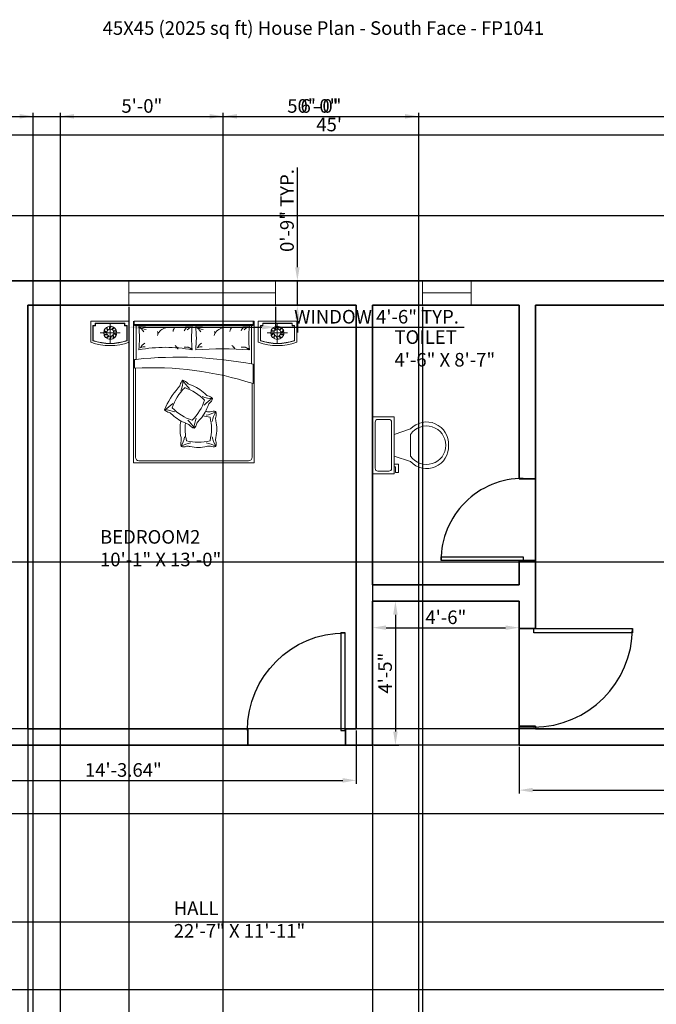
# Model space of a CAD drawing. Units: inches. Extents: x -938 to -211, y -366 to 366.
# Tile 3 of 4: x -684 to -450, y 4 to 366. Entities that reach past the tile are written whole.
import ezdxf

# ---------------------------------------------------------------- set-up
doc = ezdxf.new("R2010")
doc.units = ezdxf.units.IN
doc.header["$PDMODE"] = 35
doc.header["$PDSIZE"] = 5
for name, color, linetype, lineweight in [('A-ANNO-DIMS', 2, 'Continuous', 18), ('A-AREA-IDEN', 7, 'Continuous', 18), ('A-DOOR', 3, 'Continuous', 25), ('A-FLOR-FIXT', 9, 'Continuous', 18), ('A-GLAZ', 4, 'Continuous', 18), ('A-WALL', 7, 'Continuous', 35), ('C-PROP', 8, 'Continuous', 25), ('furn', 28, 'Continuous', 13), ('txt', 7, 'Continuous', 18)]:
    doc.layers.add(name, color=color, linetype=linetype, lineweight=lineweight)
doc.styles.get("Standard").update_dxf_attribs({"font": 'arial.ttf'})
doc.dimstyles.new('ISO-25', dxfattribs={"dimtxt": 5, "dimasz": 5, "dimexe": 1.25, "dimexo": 0.625, "dimtad": 1, "dimlunit": 3, "dimtxsty": 'Standard', "dimcen": 2.5, "dimadec": 0, "dimazin": 0, "dimtfac": 1, "dimtmove": 0, "dimatfit": 3, "dimfxl": 1, "dimarcsym": 0})

# ---------------------------------------------------------------- blocks, each defined once
blk = doc.blocks.new('*U2')
for p, q in [((0, 0), (0, -6)), ((40, 0), (40, -6))]:
    blk.add_line(p, q)
blk.add_lwpolyline([(0, 0), (0, 40), (1.75, 40), (1.75, 0)], close=True)
blk.add_arc((0, 0), 40, 0, 90)
blk = doc.blocks.new('*U4')
for p, q in [((9.5, -6), (9.5, -2)), ((-10, -8.5), (-8, -8.5)), ((-10, -9.5), (-10, -8.5)), ((-7, -9.5), (-10, -9.5)), ((-8, -8.5), (-8, -8)), ((-7, -8), (-7, -9.5)), ((-4, -8), (-6, -14)), ((4, -8), (6, -14)), ((4, -14), (-4, -14))]:
    blk.add_line(p, q)
blk.add_lwpolyline([(10.5, -8), (10.5, 0), (-10.5, 0), (-10.5, -8)], close=True)
for points in [[(-9.5, -2), (-9.5, -6)], [(8.5, -1), (-8.5, -1)], [(-8.5, -7), (8.5, -7)]]:
    blk.add_lwpolyline(points)
for centre, radius, start, end in [((-8.625, -1.875), 0.8839, 81.8699, 188.1301), ((8.625, -1.875), 0.8839, 351.8699, 98.1301), ((-8.625, -6.125), 0.8839, 171.869898, 278.1301), ((8.625, -6.125), 0.8839, 261.8699, 8.1301), ((-0.4772, -19.9188), 8.0953, 133.01722, 273.38), ((0.0374, -19.8731), 7.127, 124.50543, 269.7), ((-0.0373, -19.8731), 7.127, 270.3, 55.4946), ((0.4773, -19.9188), 8.0953, 266.62, 46.9828)]:
    blk.add_arc(centre, radius, start, end)
blk = doc.blocks.new('*D7')
at = {"layer": 'A-ANNO-DIMS', "color": 0, "lineweight": -2, "transparency": 16777216}
for p, q in [((-554.06, 151.36), (-554.06, 140.97)), ((-500.06, 151.36), (-500.06, 140.97)), ((-549.06, 142.22), (-505.06, 142.22))]:
    blk.add_line(p, q, dxfattribs=at)
at = {"layer": 'A-ANNO-DIMS', "color": 0, "transparency": 16777216}
for points in [[(-549.06, 143.05), (-549.06, 141.39), (-554.06, 142.22)], [(-505.06, 143.05), (-505.06, 141.39), (-500.06, 142.22)]]:
    blk.add_solid(points, dxfattribs=at)
at = {"layer": 'Defpoints', "color": 0, "transparency": 16777216}
for p in [(-554.06, 151.98), (-500.06, 151.98), (-500.06, 142.22)]:
    blk.add_point(p, dxfattribs=at)
at = {"layer": 'A-ANNO-DIMS', "color": 0, "transparency": 16777216, "insert": (-527.06, 145.4), "char_height": 5, "attachment_point": 5}
blk.add_mtext('4\'-6"', dxfattribs=at)
blk = doc.blocks.new('*D8')
at = {"layer": 'A-ANNO-DIMS', "color": 0, "lineweight": -2, "transparency": 16777216}
for p, q in [((-553.44, 151.98), (-544.39, 151.98)), ((-545.64, 146.98), (-545.64, 103.98)), ((-553.44, 98.98), (-544.39, 98.98))]:
    blk.add_line(p, q, dxfattribs=at)
at = {"layer": 'A-ANNO-DIMS', "color": 0, "transparency": 16777216}
for points in [[(-546.47, 146.98), (-544.8, 146.98), (-545.64, 151.98)], [(-546.47, 103.98), (-544.8, 103.98), (-545.64, 98.98)]]:
    blk.add_solid(points, dxfattribs=at)
at = {"layer": 'Defpoints', "color": 0, "transparency": 16777216}
for p in [(-554.06, 151.98), (-554.06, 98.98), (-545.64, 98.98)]:
    blk.add_point(p, dxfattribs=at)
at = {"layer": 'A-ANNO-DIMS', "color": 0, "transparency": 16777216, "insert": (-548.8, 125.48), "char_height": 5, "attachment_point": 5, "rotation": 90}
blk.add_mtext('4\'-5"', dxfattribs=at)
blk = doc.blocks.new('*D9')
at = {"layer": 'A-ANNO-DIMS', "color": 0, "lineweight": -2, "transparency": 16777216}
for p, q in [((-500.06, 98.36), (-500.06, 81.14)), ((-309.06, 98.36), (-309.06, 81.14)), ((-495.06, 82.39), (-314.06, 82.39))]:
    blk.add_line(p, q, dxfattribs=at)
at = {"layer": 'A-ANNO-DIMS', "color": 0, "transparency": 16777216}
for points in [[(-495.06, 83.22), (-495.06, 81.55), (-500.06, 82.39)], [(-314.06, 83.22), (-314.06, 81.55), (-309.06, 82.39)]]:
    blk.add_solid(points, dxfattribs=at)
at = {"layer": 'Defpoints', "color": 0, "transparency": 16777216}
for p in [(-500.06, 98.98), (-309.06, 98.98), (-309.06, 82.39)]:
    blk.add_point(p, dxfattribs=at)
at = {"layer": 'A-ANNO-DIMS', "color": 0, "transparency": 16777216, "insert": (-404.56, 85.56), "char_height": 5, "attachment_point": 5}
blk.add_mtext('15\'-11"', dxfattribs=at)
blk = doc.blocks.new('*D14')
at = {"layer": 'A-ANNO-DIMS', "color": 0, "lineweight": -2, "transparency": 16777216}
for p, q in [((-560.06, 104.36), (-560.06, 84.74)), ((-731.7, 98.36), (-731.7, 84.74)), ((-726.7, 85.99), (-565.06, 85.99))]:
    blk.add_line(p, q, dxfattribs=at)
at = {"layer": 'A-ANNO-DIMS', "color": 0, "transparency": 16777216}
for points in [[(-726.7, 86.82), (-726.7, 85.15), (-731.7, 85.99)], [(-565.06, 86.82), (-565.06, 85.15), (-560.06, 85.99)]]:
    blk.add_solid(points, dxfattribs=at)
at = {"layer": 'Defpoints', "color": 0, "transparency": 16777216}
for p in [(-560.06, 104.98), (-731.7, 98.98), (-560.06, 85.99)]:
    blk.add_point(p, dxfattribs=at)
at = {"layer": 'A-ANNO-DIMS', "color": 0, "transparency": 16777216, "insert": (-645.88, 89.17), "char_height": 5, "attachment_point": 5}
blk.add_mtext('14\'-3.64"', dxfattribs=at)
blk = doc.blocks.new('*D22')
at = {"layer": 'A-ANNO-DIMS', "color": 0, "lineweight": -2, "transparency": 16777216}
for p, q in [((-840.06, 270.61), (-840.06, 324.96)), ((-835.06, 323.71), (-305.06, 323.71)), ((-300.06, 270.61), (-300.06, 324.96))]:
    blk.add_line(p, q, dxfattribs=at)
at = {"layer": 'A-ANNO-DIMS', "color": 0, "transparency": 16777216}
for points in [[(-835.06, 324.54), (-835.06, 322.87), (-840.06, 323.71)], [(-305.06, 324.54), (-305.06, 322.87), (-300.06, 323.71)]]:
    blk.add_solid(points, dxfattribs=at)
at = {"layer": 'Defpoints', "color": 0, "transparency": 16777216}
for p in [(-300.06, 323.71), (-840.06, 269.98), (-300.06, 269.98)]:
    blk.add_point(p, dxfattribs=at)
at = {"layer": 'A-ANNO-DIMS', "color": 0, "transparency": 16777216, "insert": (-570.06, 326.87), "char_height": 5, "attachment_point": 5}
blk.add_mtext("45'", dxfattribs=at)
blk = doc.blocks.new('BED-DOUBLE-WITH-NIGHTSTANDS')
for p, q in [((-30.77, -7.97), (-30.77, -0.55)), ((-21.46, -1.59), (21.46, -1.59)), ((-21.24, -1.21), (-21.24, -14.04)), ((21.22, -1.21), (21.22, -15.71)), ((30.77, -7.97), (30.77, -0.55)), ((-34.48, -4.26), (-27.06, -4.26)), ((34.48, -4.26), (27.06, -4.26))]:
    blk.add_line(p, q)
for points in [[(-37.91, -7.71), (-37.91, 0), (-23.78, 0), (-23.78, -7.71, -0.181818)], [(-20.26, -10.53, 0.058596), (-20.26, -1.94, 0.036889), (-0.58, -1.94, 0.052163), (-0.58, -10.53, 0.093111)], [(0.7, -10.53, 0.058596), (0.7, -1.94, 0.036648), (20.51, -1.94, 0.052163), (20.51, -10.53, 0.036967)], [(37.91, -7.71), (37.91, 0), (23.78, 0), (23.78, -7.71, 0.181818)], [(-21.84, -14.04), (-21.24, -14.04, -0.072944), (21.82, -15.84), (21.82, -22.97, 0.092568), (-21.84, -17.31)]]:
    blk.add_lwpolyline(points, format="xyb", close=True)
for points in [[(-36.29, -0.77), (-36.29, -1.62), (-37.14, -1.62)], [(-36.22, -0.77), (-36.22, -1.7), (-37.14, -1.7)], [(-36.29, -0.77), (-25.39, -0.77)], [(-36.29, -0.85), (-25.39, -0.85)], [(-25.47, -0.77), (-25.47, -1.7), (-24.55, -1.7)], [(-25.39, -0.77), (-25.39, -1.62), (-24.55, -1.62)], [(-22.23, 0), (-22.23, -52.18), (22.23, -52.18), (22.23, 0)], [(21.82, 0), (21.82, -1.21), (-21.98, -1.21), (-21.98, 0), (22.23, 0)], [(25.39, -0.77), (25.39, -1.62), (24.55, -1.62)], [(25.47, -0.77), (25.47, -1.7), (24.55, -1.7)], [(36.29, -0.77), (25.39, -0.77)], [(36.29, -0.85), (25.39, -0.85)], [(36.22, -0.77), (36.22, -1.7), (37.14, -1.7)], [(36.29, -0.77), (36.29, -1.62), (37.14, -1.62)]]:
    blk.add_lwpolyline(points)
for points in [[(-24.55, -1.62), (-24.55, -7.18, -0.167087), (-37.14, -7.18), (-37.14, -1.62)], [(-24.62, -1.62), (-24.62, -7.12, -0.165559), (-37.06, -7.12), (-37.06, -1.62)], [(24.55, -1.62), (24.55, -7.17, 0.167087), (37.14, -7.17), (37.14, -1.62)], [(24.62, -1.62), (24.62, -7.12, 0.165559), (37.06, -7.12), (37.06, -1.62)], [(-21.46, -17.29), (-21.46, -50.12, 0.414214), (-20.18, -51.41), (20.18, -51.41, 0.414214), (21.46, -50.12), (21.46, -22.84)], [(-4.77, -25.48, 0.091296), (-3.99, -21.71, 0.091296), (-1.62, -24.74, 0.091296)], [(-7.96, -31.91, 0.111006), (-0.61, -36.48, 0.119549), (4.01, -29.05, 0.107813), (-3.31, -24.46)], [(-3.34, -24.47, 0.121865), (-7.96, -31.91, 0.121865)], [(0.12, -39.42, 0.159461), (1.12, -37.65, -0.076283), (1.91, -36.55, 0.115075), (5.13, -31.37, -0.076283), (5.77, -30.18, 0.159461), (6.92, -28.51)], [(3.15, -27.72, 0.091296), (6.92, -28.51, 0.091296), (3.88, -30.87, 0.091296)], [(-7.02, -33.41, 0.091296), (-10.79, -32.62, 0.091296), (-7.75, -30.26, 0.091296)], [(-2.67, -44.06, 0.111006), (5.98, -44.05, 0.119549), (5.98, -35.3, 0.033212), (3.32, -34.89)], [(0.9, -35.65, 0.091296), (0.12, -39.42, 0.091296), (-2.25, -36.39)], [(4.54, -34.62, 0.091296), (8.15, -33.3, 0.091296), (6.83, -36.91, 0.091296)], [(8.15, -46.15, 0.159461), (8.07, -44.13, -0.076283), (8.15, -42.78, 0.115075), (8.15, -36.68, -0.076283), (8.07, -35.33, 0.159461), (8.15, -33.3)], [(-1.08, -44.84, 0.091296), (-4.7, -46.15, 0.091296), (-3.37, -42.55, 0.091296)], [(6.83, -42.55, 0.091296), (8.15, -46.15, 0.091296), (4.54, -44.84)]]:
    blk.add_lwpolyline(points, format="xyb")
for centre, radius in [((-30.77, -4.26), 2.42), ((-30.77, -4.26), 1.31), ((30.77, -4.26), 2.42), ((30.77, -4.26), 1.31)]:
    blk.add_circle(centre, radius)
for centre, radius, start, end in [((-31.66, -2.67), 1.56, 208.17, 254.4897), ((-31.77, -2.78), 1.19, 196.3002, 256.538), ((-30.56, -2.45), 1.56, 172.17, 218.4897), ((-30.71, -2.48), 1.19, 160.3002, 220.538), ((-29.53, -2.92), 1.56, 136.17, 182.4897), ((-29.67, -2.86), 1.19, 124.3002, 184.538), ((-28.98, -3.9), 1.56, 100.17, 146.4897), ((-29.06, -3.77), 1.19, 88.3002, 148.538), ((-29.11, -5.02), 1.56, 64.17, 110.4897), ((-21.46, -0.82), 0.771, 180, 270), ((-15.69, 5.24), 8.51, 237.5379, 257.5233), ((-26.7, -9.98), 10.3, 36.4935, 51.2792), ((-9.16, -7.04), 4.76, 96.6849, 148.3182), ((-4.35, -4.33), 3.34, 141.8174, 169.8987), ((-0.12, -4.8), 3.6, 130.5354, 160.3558), ((2.12, -7.83), 6.48, 114.6457, 134.1585), ((-5.74, -9.98), 10.3, 36.4935, 51.2792), ((5.27, 5.24), 8.51, 237.5379, 257.5233), ((11.8, -7.04), 4.76, 96.6849, 148.3182), ((16.61, -4.33), 3.34, 141.8174, 169.8987), ((20.84, -4.8), 3.6, 130.5354, 160.3558), ((23.08, -7.83), 6.48, 114.6457, 134.1585), ((21.46, -0.82), 0.771, 270, 0), ((29.11, -5.03), 1.56, 69.5103, 115.83), ((29.06, -3.77), 1.19, 31.462, 91.6998), ((28.98, -3.9), 1.56, 33.5103, 79.83), ((29.67, -2.86), 1.19, 355.462, 55.6998), ((29.53, -2.92), 1.56, 357.5103, 43.83), ((30.71, -2.48), 1.19, 319.462, 19.6998), ((30.73, -2.38), 1.56, 321.5103, 7.83), ((31.94, -2.72), 1.19, 283.462, 343.6998), ((31.84, -2.6), 1.56, 285.5103, 331.83), ((-32.44, -3.65), 1.19, 232.3002, 292.538), ((-32.43, -3.5), 1.56, 244.17, 290.4897), ((-32.48, -4.75), 1.19, 268.3002, 328.538), ((-32.56, -4.62), 1.56, 280.17, 326.4897), ((-31.87, -5.66), 1.19, 304.3002, 4.538), ((-32.01, -5.6), 1.56, 316.17, 2.4897), ((-30.83, -6.04), 1.19, 340.3002, 40.538), ((-30.99, -6.07), 1.56, 352.17, 38.4897), ((-29.1, -4.87), 1.19, 52.3002, 112.538), ((-29.78, -5.74), 1.19, 16.3002, 76.538), ((-29.88, -5.85), 1.56, 28.17, 74.4897), ((-15.35, -4.38), 2.13, 335.8927, 16.1192), ((5.61, -4.38), 2.13, 335.8927, 16.1192), ((29.1, -4.87), 1.19, 67.462, 127.6998), ((29.88, -5.85), 1.56, 105.5103, 151.83), ((29.78, -5.74), 1.19, 103.462, 163.6998), ((30.99, -6.07), 1.56, 141.5103, 187.83), ((30.83, -6.04), 1.19, 139.462, 199.6998), ((32.01, -5.6), 1.56, 177.5103, 223.83), ((31.87, -5.66), 1.19, 175.462, 235.6998), ((32.56, -4.62), 1.56, 213.5103, 259.83), ((32.48, -4.75), 1.19, 211.462, 271.6998), ((32.61, -3.43), 1.56, 249.5103, 295.83), ((32.62, -3.58), 1.19, 247.462, 307.6998), ((-16.88, -10.73), 2.86, 114.2916, 160.9896), ((-18.36, -11.33), 1.95, 76.4823, 128.5563), ((-14.47, -16.51), 10.73, 36.2085, 45.0849), ((-6.53, -10.17), 0.72, 353.7543, 77.2187), ((-3.09, -12.99), 3.51, 44.406, 96.8342), ((-2.43, -11.76), 2.23, 33.6349, 90.8456), ((4.08, -10.73), 2.86, 114.2916, 160.9896), ((2.6, -11.33), 1.95, 76.4823, 128.5563), ((6.49, -16.51), 10.73, 36.2085, 45.0849), ((14.43, -10.17), 0.72, 353.7543, 77.2187), ((17.87, -12.99), 3.51, 44.406, 96.8342), ((18.53, -11.76), 2.23, 33.6349, 90.8456), ((-1.79, -24.12), 3.26, 132.4658, 168.7065), ((-4.85, -24.74), 3.14, 37.2937, 74.0973), ((15.27, -43.27), 28.15, 138.3818, 157.7644), ((-8.96, -21.45), 4.46, 315.5854, 333.0343), ((0.32, -19.25), 4.46, 233.2983, 250.7472), ((-5.44, -36.19), 13.43, 45.1307, 71.3884), ((7.15, -23.48), 4.46, 225.7718, 243.2208), ((4.59, -30.42), 3.01, 39.4726, 79.6505), ((-8.39, -30.41), 3.26, 222.6522, 258.8929), ((-11.03, -37.59), 4.46, 45.7718, 63.2208), ((1.56, -24.88), 13.43, 225.1307, 251.3884), ((1.73, -46.36), 13.43, 77.0576, 78.7033), ((5.69, -28.91), 4.46, 257.6988, 275.1477), ((7.19, -36.15), 3.01, 71.3996, 111.5774), ((8.38, -39.73), 13.43, 166.8711, 193.1289), ((15.01, -39.64), 18.22, 173.1956, 194.0284), ((-4.2, -41.82), 4.46, 53.2983, 70.7472), ((1.37, -35.91), 3.73, 218.7754, 250.3571), ((-9.05, -43.74), 4.46, 355.0387, 12.4877), ((-1.56, -45.28), 3.26, 159.3666, 195.6073), ((-3.83, -43.01), 3.26, 254.5791, 290.8198), ((-2.27, -50.5), 4.46, 77.6988, 95.1477), ((1.69, -33.06), 13.43, 257.0576, 283.3153), ((5.76, -50.48), 4.46, 85.2252, 102.6741), ((7.36, -42.51), 3.73, 250.7023, 282.284)]:
    blk.add_arc(centre, radius, start, end)
blk = doc.blocks.new('WINDOW-54IN')
blk.add_line((54, 0), (0, 0))
blk.add_lwpolyline([(54, 4.5), (54, -4.5), (0, -4.5), (0, 4.5)], close=True)
blk = doc.blocks.new('WINDOW-18IN')
blk.add_line((18, 0), (0, 0))
blk.add_lwpolyline([(18, 4.5), (18, -4.5), (0, -4.5), (0, 4.5)], close=True)
blk = doc.blocks.new('*D31')
at = {"layer": 'A-ANNO-DIMS', "color": 0, "lineweight": -2, "transparency": 16777216}
for p, q in [((-643.86, 260.36), (-643.86, 251.63)), ((-589.86, 260.36), (-589.86, 251.63)), ((-638.86, 252.88), (-594.86, 252.88)), ((-589.86, 252.88), (-520.34, 252.88))]:
    blk.add_line(p, q, dxfattribs=at)
at = {"layer": 'A-ANNO-DIMS', "color": 0, "transparency": 16777216}
for points in [[(-638.86, 253.72), (-638.86, 252.05), (-643.86, 252.88)], [(-594.86, 253.72), (-594.86, 252.05), (-589.86, 252.88)]]:
    blk.add_solid(points, dxfattribs=at)
at = {"layer": 'Defpoints', "color": 0, "transparency": 16777216}
for p in [(-643.86, 260.98), (-589.86, 260.98), (-589.86, 252.88)]:
    blk.add_point(p, dxfattribs=at)
at = {"layer": 'A-ANNO-DIMS', "color": 0, "transparency": 16777216, "insert": (-552.6, 256.09), "char_height": 5, "attachment_point": 5}
blk.add_mtext('WINDOW 4\'-6" TYP.', dxfattribs=at)
blk = doc.blocks.new('*D32')
at = {"layer": 'A-ANNO-DIMS', "color": 0, "lineweight": -2, "transparency": 16777216}
for p, q in [((-581.76, 274.98), (-581.76, 311.71)), ((-589.23, 269.98), (-580.51, 269.98)), ((-581.76, 260.98), (-581.76, 269.98)), ((-589.23, 260.98), (-580.51, 260.98)), ((-581.76, 255.98), (-581.76, 250.98))]:
    blk.add_line(p, q, dxfattribs=at)
at = {"layer": 'A-ANNO-DIMS', "color": 0, "transparency": 16777216}
for points in [[(-582.59, 274.98), (-580.93, 274.98), (-581.76, 269.98)], [(-582.59, 255.98), (-580.93, 255.98), (-581.76, 260.98)]]:
    blk.add_solid(points, dxfattribs=at)
at = {"layer": 'Defpoints', "color": 0, "transparency": 16777216}
for p in [(-589.86, 269.98), (-581.76, 269.98), (-589.86, 260.98)]:
    blk.add_point(p, dxfattribs=at)
at = {"layer": 'A-ANNO-DIMS', "color": 0, "transparency": 16777216, "insert": (-584.94, 295.85), "char_height": 5, "attachment_point": 5, "rotation": 90}
blk.add_mtext('0\'-9" TYP.', dxfattribs=at)
blk = doc.blocks.new('*D43')
at = {"layer": 'A-ANNO-DIMS', "color": 0, "lineweight": -2, "transparency": 16777216}
for p, q in [((-876.06, 294.61), (-876.06, 331.78)), ((-871.06, 330.53), (-281.06, 330.53)), ((-276.06, 294.61), (-276.06, 331.78))]:
    blk.add_line(p, q, dxfattribs=at)
at = {"layer": 'A-ANNO-DIMS', "color": 0, "transparency": 16777216}
for points in [[(-871.06, 331.37), (-871.06, 329.7), (-876.06, 330.53)], [(-281.06, 331.37), (-281.06, 329.7), (-276.06, 330.53)]]:
    blk.add_solid(points, dxfattribs=at)
at = {"layer": 'Defpoints', "color": 0, "transparency": 16777216}
for p in [(-276.06, 330.53), (-876.06, 293.98), (-276.06, 293.98)]:
    blk.add_point(p, dxfattribs=at)
at = {"layer": 'A-ANNO-DIMS', "color": 0, "transparency": 16777216, "insert": (-576.06, 333.71), "char_height": 5, "attachment_point": 5}
blk.add_mtext('50\'-0"', dxfattribs=at)
blk = doc.blocks.new('*D45')
at = {"layer": 'A-ANNO-DIMS', "color": 0, "lineweight": -2, "transparency": 16777216}
for p, q in [((-609.06, -227.28), (-609.06, 331.78)), ((-604.06, 330.53), (-542.06, 330.53)), ((-537.06, -227.28), (-537.06, 331.78))]:
    blk.add_line(p, q, dxfattribs=at)
at = {"layer": 'A-ANNO-DIMS', "color": 0, "transparency": 16777216}
for points in [[(-604.06, 331.37), (-604.06, 329.7), (-609.06, 330.53)], [(-542.06, 331.37), (-542.06, 329.7), (-537.06, 330.53)]]:
    blk.add_solid(points, dxfattribs=at)
at = {"layer": 'Defpoints', "color": 0, "transparency": 16777216}
for p in [(-537.06, 330.53), (-609.06, -227.9), (-537.06, -227.9)]:
    blk.add_point(p, dxfattribs=at)
at = {"layer": 'A-ANNO-DIMS', "color": 0, "transparency": 16777216, "insert": (-573.06, 333.71), "char_height": 5, "attachment_point": 5}
blk.add_mtext('6\'-0"', dxfattribs=at)
blk = doc.blocks.new('*D47')
at = {"layer": 'A-ANNO-DIMS', "color": 0, "lineweight": -2, "transparency": 16777216}
for p, q in [((-715.02, -44.58), (-715.02, 331.78)), ((-710.02, 330.53), (-684.06, 330.53)), ((-679.06, -44.58), (-679.06, 331.78))]:
    blk.add_line(p, q, dxfattribs=at)
at = {"layer": 'A-ANNO-DIMS', "color": 0, "transparency": 16777216}
for points in [[(-710.02, 331.37), (-710.02, 329.7), (-715.02, 330.53)], [(-684.06, 331.37), (-684.06, 329.7), (-679.06, 330.53)]]:
    blk.add_solid(points, dxfattribs=at)
at = {"layer": 'Defpoints', "color": 0, "transparency": 16777216}
for p in [(-679.06, 330.53), (-715.02, -45.21), (-679.06, -45.21)]:
    blk.add_point(p, dxfattribs=at)
at = {"layer": 'A-ANNO-DIMS', "color": 0, "transparency": 16777216, "insert": (-697.04, 333.71), "char_height": 5, "attachment_point": 5}
blk.add_mtext('3\'-0"', dxfattribs=at)
blk = doc.blocks.new('*D49')
at = {"layer": 'A-ANNO-DIMS', "color": 0, "lineweight": -2, "transparency": 16777216}
for p, q in [((-669.06, -260.39), (-669.06, 331.78)), ((-664.06, 330.53), (-614.06, 330.53)), ((-609.06, -260.39), (-609.06, 331.78))]:
    blk.add_line(p, q, dxfattribs=at)
at = {"layer": 'A-ANNO-DIMS', "color": 0, "transparency": 16777216}
for points in [[(-664.06, 331.37), (-664.06, 329.7), (-669.06, 330.53)], [(-614.06, 331.37), (-614.06, 329.7), (-609.06, 330.53)]]:
    blk.add_solid(points, dxfattribs=at)
at = {"layer": 'Defpoints', "color": 0, "transparency": 16777216}
for p in [(-609.06, 330.53), (-669.06, -261.02), (-609.06, -261.02)]:
    blk.add_point(p, dxfattribs=at)
at = {"layer": 'A-ANNO-DIMS', "color": 0, "transparency": 16777216, "insert": (-639.06, 333.71), "char_height": 5, "attachment_point": 5}
blk.add_mtext('5\'-0"', dxfattribs=at)
blk = doc.blocks.new('*D56')
at = {"layer": 'A-ANNO-DIMS', "color": 0, "lineweight": -2, "transparency": 16777216}
for p, q in [((-309.69, 166.31), (-928.86, 166.31)), ((-927.61, 109.98), (-927.61, 161.31)), ((-309.69, 104.98), (-928.86, 104.98))]:
    blk.add_line(p, q, dxfattribs=at)
at = {"layer": 'A-ANNO-DIMS', "color": 0, "transparency": 16777216}
for points in [[(-928.45, 161.31), (-926.78, 161.31), (-927.61, 166.31)], [(-928.45, 109.98), (-926.78, 109.98), (-927.61, 104.98)]]:
    blk.add_solid(points, dxfattribs=at)
at = {"layer": 'Defpoints', "color": 0, "transparency": 16777216}
for p in [(-927.61, 166.31), (-309.06, 166.31), (-309.06, 104.98)]:
    blk.add_point(p, dxfattribs=at)
at = {"layer": 'A-ANNO-DIMS', "color": 0, "transparency": 16777216, "insert": (-930.82, 135.65), "char_height": 5, "attachment_point": 5, "rotation": 90}
blk.add_mtext('5\'-1 1/2"', dxfattribs=at)
blk = doc.blocks.new('*D57')
at = {"layer": 'A-ANNO-DIMS', "color": 0, "lineweight": -2, "transparency": 16777216}
for p, q in [((-681.06, 260.36), (-681.06, -363.01)), ((-643.86, 260.36), (-643.86, -363.01)), ((-648.86, -361.76), (-676.06, -361.76))]:
    blk.add_line(p, q, dxfattribs=at)
at = {"layer": 'A-ANNO-DIMS', "color": 0, "transparency": 16777216}
for points in [[(-676.06, -360.93), (-676.06, -362.6), (-681.06, -361.76)], [(-648.86, -360.93), (-648.86, -362.6), (-643.86, -361.76)]]:
    blk.add_solid(points, dxfattribs=at)
at = {"layer": 'Defpoints', "color": 0, "transparency": 16777216}
for p in [(-681.06, 260.98), (-643.86, 260.98), (-681.06, -361.76)]:
    blk.add_point(p, dxfattribs=at)
at = {"layer": 'A-ANNO-DIMS', "color": 0, "transparency": 16777216, "insert": (-662.46, -358.58), "char_height": 5, "attachment_point": 5}
blk.add_mtext('3\'-1"', dxfattribs=at)
blk = doc.blocks.new('*D58')
at = {"layer": 'A-ANNO-DIMS', "color": 0, "lineweight": -2, "transparency": 16777216}
for p, q in [((-554.06, 260.36), (-554.06, -363.01)), ((-535.69, 260.36), (-535.69, -363.01)), ((-554.06, -361.76), (-584.78, -361.76)), ((-540.69, -361.76), (-549.06, -361.76))]:
    blk.add_line(p, q, dxfattribs=at)
at = {"layer": 'A-ANNO-DIMS', "color": 0, "transparency": 16777216}
for points in [[(-549.06, -360.93), (-549.06, -362.6), (-554.06, -361.76)], [(-540.69, -360.93), (-540.69, -362.6), (-535.69, -361.76)]]:
    blk.add_solid(points, dxfattribs=at)
at = {"layer": 'Defpoints', "color": 0, "transparency": 16777216}
for p in [(-554.06, 260.98), (-535.69, 260.98), (-554.06, -361.76)]:
    blk.add_point(p, dxfattribs=at)
at = {"layer": 'A-ANNO-DIMS', "color": 0, "transparency": 16777216, "insert": (-571.92, -358.55), "char_height": 5, "attachment_point": 5}
blk.add_mtext('1\'-6 1/2"', dxfattribs=at)
blk = doc.blocks.new('*D60')
at = {"layer": 'A-ANNO-DIMS', "color": 0, "lineweight": -2, "transparency": 16777216}
for p, q in [((-394.97, 33.71), (-928.86, 33.71)), ((-927.61, 28.71), (-927.61, 13.79)), ((-418.97, 8.79), (-928.86, 8.79))]:
    blk.add_line(p, q, dxfattribs=at)
at = {"layer": 'A-ANNO-DIMS', "color": 0, "transparency": 16777216}
for points in [[(-928.45, 28.71), (-926.78, 28.71), (-927.61, 33.71)], [(-928.45, 13.79), (-926.78, 13.79), (-927.61, 8.79)]]:
    blk.add_solid(points, dxfattribs=at)
at = {"layer": 'Defpoints', "color": 0, "transparency": 16777216}
for p in [(-394.34, 33.71), (-927.61, 8.79), (-418.34, 8.79)]:
    blk.add_point(p, dxfattribs=at)
at = {"layer": 'A-ANNO-DIMS', "color": 0, "transparency": 16777216, "insert": (-930.75, 21.25), "char_height": 5, "attachment_point": 5, "rotation": 90}
blk.add_mtext('2\'-1"', dxfattribs=at)
blk = doc.blocks.new('*D66')
at = {"layer": 'A-ANNO-DIMS', "color": 0, "lineweight": -2, "transparency": 16777216}
for p, q in [((-309.69, 98.98), (-928.86, 98.98)), ((-927.61, 93.98), (-927.61, 78.67)), ((-309.69, 73.67), (-928.86, 73.67)), ((-927.61, 73.67), (-927.61, 42.39))]:
    blk.add_line(p, q, dxfattribs=at)
at = {"layer": 'A-ANNO-DIMS', "color": 0, "transparency": 16777216}
for points in [[(-928.45, 93.98), (-926.78, 93.98), (-927.61, 98.98)], [(-928.45, 78.67), (-926.78, 78.67), (-927.61, 73.67)]]:
    blk.add_solid(points, dxfattribs=at)
at = {"layer": 'Defpoints', "color": 0, "transparency": 16777216}
for p in [(-309.06, 98.98), (-927.61, 73.67), (-309.06, 73.67)]:
    blk.add_point(p, dxfattribs=at)
at = {"layer": 'A-ANNO-DIMS', "color": 0, "transparency": 16777216, "insert": (-930.82, 55.53), "char_height": 5, "attachment_point": 5, "rotation": 90}
blk.add_mtext('2\'-1 1/2"', dxfattribs=at)

msp = doc.modelspace()

# ---------------------------------------------------------------- linework, layer by layer
at = {"layer": 'A-WALL'}
for p, q in [((-840.062, 269.982), (-300.062, 269.982)), ((-681.062, 104.982), (-681.062, 260.982)), ((-681.062, 260.982), (-560.062, 260.982)), ((-560.062, 104.982), (-560.062, 260.982)), ((-554.062, 260.982), (-500.062, 260.982)), ((-554.062, 157.982), (-554.062, 260.982)), ((-500.062, 196.982), (-500.062, 260.982)), ((-494.062, 260.982), (-309.062, 260.982)), ((-494.062, 141.906), (-494.062, 260.982)), ((-500.062, 196.982), (-494.062, 196.982)), ((-500.062, 157.982), (-500.062, 166.982)), ((-500.062, 166.982), (-494.062, 166.982)), ((-554.062, 157.982), (-500.062, 157.982)), ((-554.062, 98.982), (-554.062, 151.982)), ((-554.062, 151.982), (-500.062, 151.982)), ((-500.062, 98.982), (-500.062, 151.982)), ((-494.062, 141.906), (-500.062, 141.906)), ((-494.062, 105.906), (-500.062, 105.906)), ((-494.062, 104.982), (-494.062, 105.906)), ((-681.062, 104.982), (-600.062, 104.982)), ((-600.062, 104.982), (-600.062, 98.982)), ((-564.062, 104.982), (-564.062, 98.982)), ((-564.062, 104.982), (-560.062, 104.982)), ((-494.062, 104.982), (-309.062, 104.982)), ((-831.062, 98.982), (-554.062, 98.982)), ((-500.062, 98.982), (-309.062, 98.982))]:
    msp.add_line(p, q, dxfattribs=at)
at = {"layer": 'C-PROP'}
msp.add_line((-876.062, 293.982), (-300.062, 293.982), dxfattribs=at)

# ---------------------------------------------------------------- block references
at = {"layer": 'A-DOOR'}
for p, xscale, yscale, zscale, rotation in [((-498.598, 166.982), 0.7558877724910423, 0.7558877724910423, 0.7558877724910423, 89.99999999999996), ((-494.622, 141.906), 0.9067907245945414, 0.9067907245945414, 0.9067907245945414, 270)]:
    msp.add_blockref('*U2', p, dxfattribs=dict(at, xscale=xscale, yscale=yscale, zscale=zscale, rotation=rotation))
at = {"layer": 'A-DOOR', "xscale": -0.8986880990233336, "yscale": 0.8986880990233336, "zscale": 0.8986880990233336}
msp.add_blockref('*U2', (-564.214, 104.374), dxfattribs=at)
at = {"layer": 'A-FLOR-FIXT', "rotation": 90}
msp.add_blockref('*U4', (-554.062, 209.407), dxfattribs=at)
at = {"layer": 'A-GLAZ'}
for name, p in [('WINDOW-54IN', (-643.859, 265.482)), ('WINDOW-18IN', (-535.694, 265.482))]:
    msp.add_blockref(name, p, dxfattribs=at)
at = {"layer": 'furn'}
msp.add_blockref('BED-DOUBLE-WITH-NIGHTSTANDS', (-619.929, 255.079), dxfattribs=at)

# ---------------------------------------------------------------- texts
at = {"layer": 'A-AREA-IDEN', "char_height": 5, "attachment_point": 1}
for s, width, insert in [('TOILET\\P4\'-6" X 8\'-7"', 39.42684, (-545.987, 251.733)), ('BEDROOM2\\P10\'-1" X 13\'-0"', 72.52243, (-654.472, 178.159)), ('HALL\\P22\'-7" X 11\'-11"', 103.96102, (-627.323, 41.412))]:
    msp.add_mtext_dynamic_manual_height_columns(s, width=width, gutter_width=12.5, heights=[0], dxfattribs=dict(at, insert=insert))
at = {"layer": 'txt', "insert": (-653.517, 365.548), "char_height": 5, "attachment_point": 1}
msp.add_mtext_dynamic_manual_height_columns('45X45 (2025 sq ft) House Plan - South Face - FP1041', width=564.69648, gutter_width=12.5, heights=[0], dxfattribs=at)

# ---------------------------------------------------------------- dimensions: what is measured, and where the dimension line sits
at = {"layer": 'A-ANNO-DIMS'}
for base, p1, p2, override, picture, middle in [((-276.062, 330.532), (-876.062, 293.982), (-276.062, 293.982), {"dimdec": 1, "dimlfac": 1, "dimrnd": 0, "dimzin": 1, "dimdsep": 46, "dimlunit": 4, "dimfrac": 2}, '*D43', (-576.062, 333.71)), ((-679.062, 330.532), (-715.024, -45.209), (-679.062, -45.209), {"dimdec": 1, "dimlfac": 1, "dimrnd": 0, "dimzin": 1, "dimdsep": 46, "dimlunit": 4, "dimfrac": 2}, '*D47', (-697.043, 333.711)), ((-609.062, 330.532), (-669.062, -261.018), (-609.062, -261.018), {"dimdec": 1, "dimlfac": 1, "dimrnd": 0, "dimzin": 1, "dimdsep": 46, "dimlunit": 4, "dimfrac": 2}, '*D49', (-639.062, 333.71)), ((-537.062, 330.532), (-609.062, -227.9), (-537.062, -227.9), {"dimdec": 1, "dimlfac": 1, "dimrnd": 0, "dimzin": 1, "dimdsep": 46, "dimlunit": 4, "dimfrac": 2}, '*D45', (-573.062, 333.71)), ((-300.062, 323.707), (-840.062, 269.982), (-300.062, 269.982), {"dimclrd": 0, "dimclre": 0, "dimclrt": 0}, '*D22', (-570.062, 326.874)), ((-681.062, -361.763), (-643.859, 260.982), (-681.062, 260.982), {"dimdec": 1, "dimlfac": 1, "dimrnd": 0, "dimzin": 1, "dimdsep": 46, "dimlunit": 4, "dimfrac": 2}, '*D57', (-662.461, -358.584)), ((-554.062, -361.763), (-535.694, 260.982), (-554.062, 260.982), {"dimdec": 1, "dimlfac": 1, "dimrnd": 0, "dimzin": 1, "dimdsep": 46, "dimlunit": 4, "dimfrac": 2}, '*D58', (-571.923, -358.553)), ((-500.062, 142.219), (-554.062, 151.982), (-500.062, 151.982), {"dimclrd": 0, "dimclre": 0, "dimclrt": 0}, '*D7', (-527.062, 145.397)), ((-560.062, 85.986), (-731.701, 98.982), (-560.062, 104.982), {"dimclrd": 0, "dimclre": 0, "dimclrt": 0}, '*D14', (-645.882, 89.166)), ((-309.062, 82.385), (-500.062, 98.982), (-309.062, 98.982), {"dimclrd": 0, "dimclre": 0, "dimclrt": 0}, '*D9', (-404.562, 85.563))]:
    dim = msp.add_linear_dim(base=base, p1=p1, p2=p2, dimstyle='ISO-25', override=override, dxfattribs=at)
    dim.commit()
    dim.dimension.update_dxf_attribs({"geometry": picture, "text_midpoint": middle})
dim = msp.add_linear_dim(base=(-581.759, 269.982), p1=(-589.859, 260.982), p2=(-589.859, 269.982), angle=90, text='<> TYP.', dimstyle='ISO-25', override={"dimdec": 1, "dimlfac": 1, "dimrnd": 0, "dimzin": 1, "dimdsep": 46, "dimlunit": 4, "dimfrac": 2}, dxfattribs=at)
dim.commit()
dim.dimension.update_dxf_attribs({"geometry": '*D32', "text_midpoint": (-584.937, 295.846)})
dim = msp.add_linear_dim(base=(-589.859, 252.882), p1=(-643.859, 260.982), p2=(-589.859, 260.982), text='WINDOW <> TYP.', dimstyle='ISO-25', override={"dimdec": 1, "dimlfac": 1, "dimrnd": 0, "dimzin": 1, "dimdsep": 46, "dimlunit": 4, "dimfrac": 2}, dxfattribs=at)
dim.commit()
dim.dimension.update_dxf_attribs({"geometry": '*D31', "text_midpoint": (-552.599, 256.094)})
for base, p1, p2, override, picture, middle in [((-927.612, 166.311), (-309.062, 104.982), (-309.062, 166.311), {"dimdec": 1, "dimlfac": 1, "dimrnd": 0, "dimzin": 1, "dimdsep": 46, "dimlunit": 4, "dimfrac": 2}, '*D56', (-930.823, 135.646)), ((-545.636, 98.982), (-554.062, 151.982), (-554.062, 98.982), {"dimclrd": 0, "dimclre": 0, "dimclrt": 0}, '*D8', (-548.803, 125.482)), ((-927.612, 73.669), (-309.062, 98.982), (-309.062, 73.669), {"dimdec": 1, "dimlfac": 1, "dimrnd": 0, "dimzin": 1, "dimdsep": 46, "dimlunit": 4, "dimfrac": 2}, '*D66', (-930.823, 55.531)), ((-927.612, 8.791), (-394.341, 33.709), (-418.341, 8.791), {"dimdec": 1, "dimlfac": 1, "dimrnd": 0, "dimzin": 1, "dimdsep": 46, "dimlunit": 4, "dimfrac": 2}, '*D60', (-930.748, 21.25))]:
    dim = msp.add_linear_dim(base=base, p1=p1, p2=p2, angle=90, dimstyle='ISO-25', override=override, dxfattribs=at)
    dim.commit()
    dim.dimension.update_dxf_attribs({"geometry": picture, "text_midpoint": middle})

doc.saveas('drawing.dxf')
